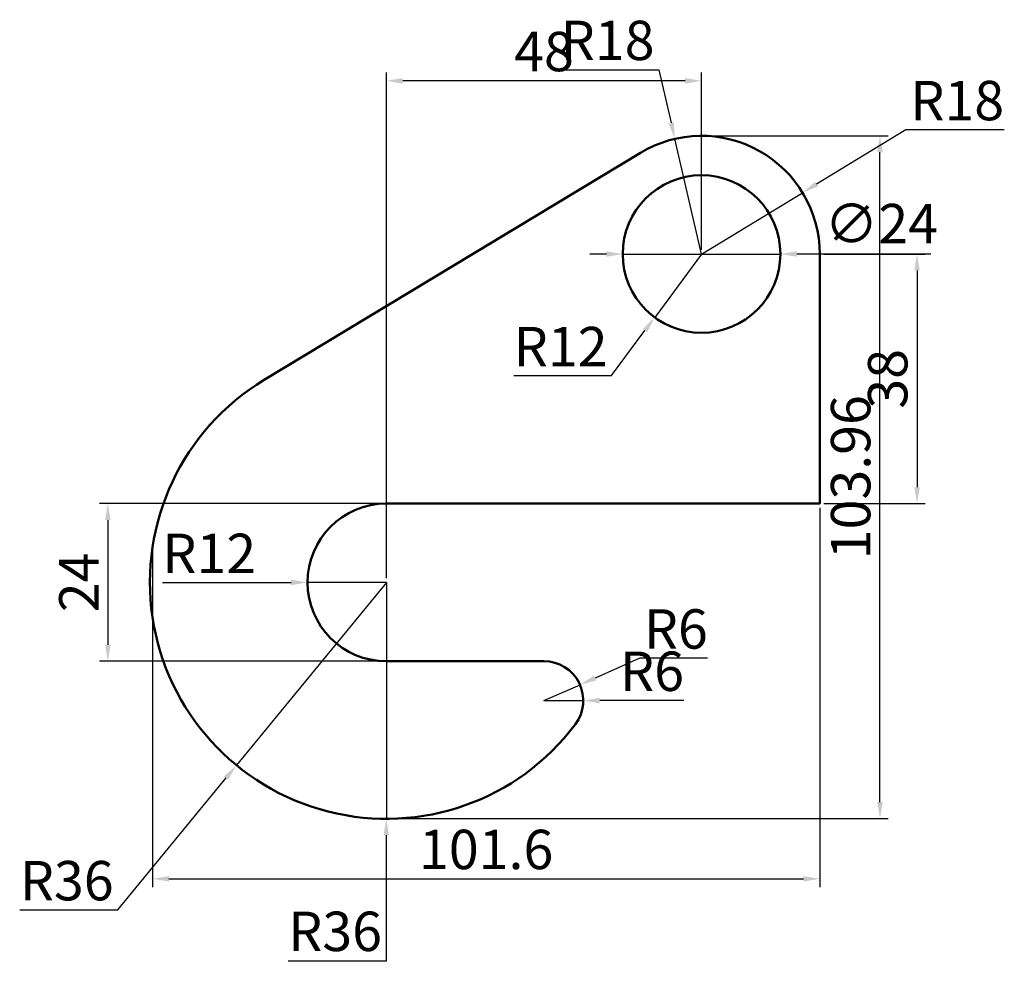
# Model space of a CAD drawing. Units: millimetres. Extents: x 135 to 285, y 18 to 161.
import ezdxf

# ---------------------------------------------------------------- set-up
doc = ezdxf.new("R2010")
doc.units = ezdxf.units.MM
doc.layers.add('M-DIMS', color=2, linetype='Continuous', lineweight=25)
doc.layers.add('M-OUTL', color=7, linetype='Continuous', lineweight=50)
doc.styles.get("Standard").update_dxf_attribs({"font": 'arial.ttf'})
doc.dimstyles.new('ISO-25', dxfattribs={"dimtxt": 6, "dimasz": 2.5, "dimexe": 1.25, "dimexo": 0.625, "dimtad": 1, "dimtoh": 1, "dimdec": 0, "dimtxsty": 'Standard', "dimcen": 2.5, "dimadec": 0, "dimazin": 0, "dimtfac": 1, "dimtdec": 0, "dimtmove": 0, "dimatfit": 3, "dimfxl": 1, "dimarcsym": 0})

# ---------------------------------------------------------------- blocks, each defined once
blk = doc.blocks.new('*D1')
at = {"layer": 'Defpoints', "color": 0, "transparency": 16777216}
for p in [(191.17, 87.46), (148.76, 63.46), (191.17, 63.46)]:
    blk.add_point(p, dxfattribs=at)
at = {"layer": 'M-DIMS', "color": 0, "lineweight": -2, "transparency": 16777216}
for p, q in [((190.54, 87.46), (147.51, 87.46)), ((148.76, 84.96), (148.76, 65.96)), ((190.54, 63.46), (147.51, 63.46))]:
    blk.add_line(p, q, dxfattribs=at)
at = {"layer": 'M-DIMS', "color": 0, "transparency": 16777216}
for points in [[(148.34, 84.96), (149.18, 84.96), (148.76, 87.46)], [(148.34, 65.96), (149.18, 65.96), (148.76, 63.46)]]:
    blk.add_solid(points, dxfattribs=at)
at = {"layer": 'M-DIMS', "color": 0, "transparency": 16777216, "insert": (145.12, 75.46), "char_height": 6, "attachment_point": 5, "rotation": 90}
blk.add_mtext('24', dxfattribs=at)
blk = doc.blocks.new('*D2')
at = {"layer": 'Defpoints', "color": 0, "transparency": 16777216}
for p in [(191.17, 75.46), (168.35, 47.61)]:
    blk.add_point(p, dxfattribs=at)
at = {"layer": 'M-DIMS', "color": 0, "lineweight": -2, "transparency": 16777216}
for p, q in [((191.17, 75.46), (168.35, 47.61)), ((150.3, 25.58), (166.77, 45.68)), ((135.34, 25.58), (150.3, 25.58))]:
    blk.add_line(p, q, dxfattribs=at)
at = {"layer": 'M-DIMS', "color": 0, "transparency": 16777216}
blk.add_solid([(166.44, 45.94), (167.09, 45.42), (168.35, 47.61)], dxfattribs=at)
at = {"layer": 'M-DIMS', "color": 0, "transparency": 16777216, "insert": (142.5, 29.27), "char_height": 6, "attachment_point": 5}
blk.add_mtext('R36', dxfattribs=at)
blk = doc.blocks.new('*D3')
at = {"layer": 'Defpoints', "color": 0, "transparency": 16777216}
for p in [(191.17, 151.83), (239.17, 125.46), (191.17, 75.46)]:
    blk.add_point(p, dxfattribs=at)
at = {"layer": 'M-DIMS', "color": 0, "lineweight": -2, "transparency": 16777216}
for p, q in [((191.17, 76.09), (191.17, 153.08)), ((239.17, 126.09), (239.17, 153.08)), ((236.67, 151.83), (193.67, 151.83))]:
    blk.add_line(p, q, dxfattribs=at)
at = {"layer": 'M-DIMS', "color": 0, "transparency": 16777216}
for points in [[(193.67, 152.25), (193.67, 151.41), (191.17, 151.83)], [(236.67, 152.25), (236.67, 151.41), (239.17, 151.83)]]:
    blk.add_solid(points, dxfattribs=at)
at = {"layer": 'M-DIMS', "color": 0, "transparency": 16777216, "insert": (215.17, 155.52), "char_height": 6, "attachment_point": 5}
blk.add_mtext('48', dxfattribs=at)
blk = doc.blocks.new('*D4')
at = {"layer": 'Defpoints', "color": 0, "transparency": 16777216}
for p in [(239.17, 125.46), (232.03, 115.81)]:
    blk.add_point(p, dxfattribs=at)
at = {"layer": 'M-DIMS', "color": 0, "lineweight": -2, "transparency": 16777216}
for p, q in [((239.17, 125.46), (232.03, 115.81)), ((225.47, 106.95), (230.54, 113.8)), ((210.57, 106.95), (225.47, 106.95))]:
    blk.add_line(p, q, dxfattribs=at)
at = {"layer": 'M-DIMS', "color": 0, "transparency": 16777216}
blk.add_solid([(230.21, 114.05), (230.88, 113.56), (232.03, 115.81)], dxfattribs=at)
at = {"layer": 'M-DIMS', "color": 0, "transparency": 16777216, "insert": (217.71, 110.59), "char_height": 6, "attachment_point": 5}
blk.add_mtext('R12', dxfattribs=at)
blk = doc.blocks.new('*D5')
at = {"layer": 'Defpoints', "color": 0, "transparency": 16777216}
for p in [(254.55, 134.8), (239.17, 125.46)]:
    blk.add_point(p, dxfattribs=at)
at = {"layer": 'M-DIMS', "color": 0, "lineweight": -2, "transparency": 16777216}
for p, q in [((270.3, 144.36), (256.69, 136.1)), ((285.27, 144.36), (270.3, 144.36)), ((239.17, 125.46), (254.55, 134.8))]:
    blk.add_line(p, q, dxfattribs=at)
at = {"layer": 'M-DIMS', "color": 0, "transparency": 16777216}
blk.add_solid([(256.47, 136.46), (256.91, 135.74), (254.55, 134.8)], dxfattribs=at)
at = {"layer": 'M-DIMS', "color": 0, "transparency": 16777216, "insert": (278.1, 148.05), "char_height": 6, "attachment_point": 5}
blk.add_mtext('R18', dxfattribs=at)
blk = doc.blocks.new('*D6')
at = {"layer": 'Defpoints', "color": 0, "transparency": 16777216}
for p in [(257.17, 125.46), (257.17, 87.46), (271.98, 87.46)]:
    blk.add_point(p, dxfattribs=at)
at = {"layer": 'M-DIMS', "color": 0, "lineweight": -2, "transparency": 16777216}
for p, q in [((257.79, 125.46), (273.23, 125.46)), ((271.98, 122.96), (271.98, 89.96)), ((257.79, 87.46), (273.23, 87.46))]:
    blk.add_line(p, q, dxfattribs=at)
at = {"layer": 'M-DIMS', "color": 0, "transparency": 16777216}
for points in [[(271.57, 122.96), (272.4, 122.96), (271.98, 125.46)], [(271.57, 89.96), (272.4, 89.96), (271.98, 87.46)]]:
    blk.add_solid(points, dxfattribs=at)
at = {"layer": 'M-DIMS', "color": 0, "transparency": 16777216, "insert": (268.29, 106.46), "char_height": 6, "attachment_point": 5, "rotation": 90}
blk.add_mtext('38', dxfattribs=at)
blk = doc.blocks.new('*D7')
at = {"layer": 'Defpoints', "color": 0, "transparency": 16777216}
for p in [(220.66, 59.88), (215.17, 57.46)]:
    blk.add_point(p, dxfattribs=at)
at = {"layer": 'M-DIMS', "color": 0, "lineweight": -2, "transparency": 16777216}
for p, q in [((229.79, 63.9), (222.95, 60.89)), ((240.09, 63.9), (229.79, 63.9)), ((215.17, 57.46), (220.66, 59.88))]:
    blk.add_line(p, q, dxfattribs=at)
at = {"layer": 'M-DIMS', "color": 0, "transparency": 16777216}
blk.add_solid([(222.78, 61.27), (223.11, 60.51), (220.66, 59.88)], dxfattribs=at)
at = {"layer": 'M-DIMS', "color": 0, "transparency": 16777216, "insert": (235.25, 67.59), "char_height": 6, "attachment_point": 5}
blk.add_mtext('R6', dxfattribs=at)
blk = doc.blocks.new('*D8')
at = {"layer": 'Defpoints', "color": 0, "transparency": 16777216}
for p in [(238.9, 143.46), (266.34, 143.46), (192.93, 39.5)]:
    blk.add_point(p, dxfattribs=at)
at = {"layer": 'M-DIMS', "color": 0, "lineweight": -2, "transparency": 16777216}
for p, q in [((239.53, 143.46), (267.59, 143.46)), ((266.34, 42), (266.34, 140.96)), ((193.55, 39.5), (267.59, 39.5))]:
    blk.add_line(p, q, dxfattribs=at)
at = {"layer": 'M-DIMS', "color": 0, "transparency": 16777216}
for points in [[(265.92, 140.96), (266.76, 140.96), (266.34, 143.46)], [(265.92, 42), (266.76, 42), (266.34, 39.5)]]:
    blk.add_solid(points, dxfattribs=at)
at = {"layer": 'M-DIMS', "color": 0, "transparency": 16777216, "insert": (262.65, 91.48), "char_height": 6, "attachment_point": 5, "rotation": 90}
blk.add_mtext('103.96', dxfattribs=at)
blk = doc.blocks.new('*D9')
at = {"layer": 'Defpoints', "color": 0, "transparency": 16777216}
for p in [(257.17, 87.46), (155.57, 80.82), (257.17, 30.33)]:
    blk.add_point(p, dxfattribs=at)
at = {"layer": 'M-DIMS', "color": 0, "lineweight": -2, "transparency": 16777216}
for p, q in [((257.17, 86.84), (257.17, 29.08)), ((155.57, 80.19), (155.57, 29.08)), ((158.07, 30.33), (254.67, 30.33))]:
    blk.add_line(p, q, dxfattribs=at)
at = {"layer": 'M-DIMS', "color": 0, "transparency": 16777216}
for points in [[(158.07, 30.74), (158.07, 29.91), (155.57, 30.33)], [(254.67, 30.74), (254.67, 29.91), (257.17, 30.33)]]:
    blk.add_solid(points, dxfattribs=at)
at = {"layer": 'M-DIMS', "color": 0, "transparency": 16777216, "insert": (206.37, 34.02), "char_height": 6, "attachment_point": 5}
blk.add_mtext('101.6', dxfattribs=at)
blk = doc.blocks.new('*D10')
at = {"layer": 'Defpoints', "color": 0, "transparency": 16777216}
for p in [(235.1, 143), (239.17, 125.46)]:
    blk.add_point(p, dxfattribs=at)
at = {"layer": 'M-DIMS', "color": 0, "lineweight": -2, "transparency": 16777216}
for p, q in [((217.69, 153.52), (232.66, 153.52)), ((232.66, 153.52), (234.54, 145.43)), ((239.17, 125.46), (235.1, 143))]:
    blk.add_line(p, q, dxfattribs=at)
at = {"layer": 'M-DIMS', "color": 0, "transparency": 16777216}
blk.add_solid([(234.94, 145.53), (234.13, 145.34), (235.1, 143)], dxfattribs=at)
at = {"layer": 'M-DIMS', "color": 0, "transparency": 16777216, "insert": (224.86, 157.21), "char_height": 6, "attachment_point": 5}
blk.add_mtext('R18', dxfattribs=at)
blk = doc.blocks.new('*D11')
at = {"layer": 'Defpoints', "color": 0, "transparency": 16777216}
for p in [(227.17, 125.46), (251.17, 125.46)]:
    blk.add_point(p, dxfattribs=at)
at = {"layer": 'M-DIMS', "color": 0, "lineweight": -2, "transparency": 16777216}
for p, q in [((224.67, 125.46), (222.17, 125.46)), ((227.17, 125.46), (251.17, 125.46)), ((258.37, 125.46), (253.67, 125.46)), ((274.09, 125.46), (258.37, 125.46))]:
    blk.add_line(p, q, dxfattribs=at)
at = {"layer": 'M-DIMS', "color": 0, "transparency": 16777216}
for points in [[(224.67, 125.88), (224.67, 125.04), (227.17, 125.46)], [(253.67, 125.88), (253.67, 125.04), (251.17, 125.46)]]:
    blk.add_solid(points, dxfattribs=at)
at = {"layer": 'M-DIMS', "color": 0, "transparency": 16777216, "insert": (266.54, 129.32), "char_height": 6, "attachment_point": 5}
blk.add_mtext('∅24', dxfattribs=at)
blk = doc.blocks.new('*D12')
at = {"layer": 'Defpoints', "color": 0, "transparency": 16777216}
for p in [(179.17, 75.46), (191.17, 75.46)]:
    blk.add_point(p, dxfattribs=at)
at = {"layer": 'M-DIMS', "color": 0, "lineweight": -2, "transparency": 16777216}
for p, q in [((157.07, 75.46), (171.97, 75.46)), ((171.97, 75.46), (176.67, 75.46)), ((191.17, 75.46), (179.17, 75.46))]:
    blk.add_line(p, q, dxfattribs=at)
at = {"layer": 'M-DIMS', "color": 0, "transparency": 16777216}
blk.add_solid([(176.67, 75.88), (176.67, 75.04), (179.17, 75.46)], dxfattribs=at)
at = {"layer": 'M-DIMS', "color": 0, "transparency": 16777216, "insert": (164.2, 79.1), "char_height": 6, "attachment_point": 5}
blk.add_mtext('R12', dxfattribs=at)
blk = doc.blocks.new('*D13')
at = {"layer": 'Defpoints', "color": 0, "transparency": 16777216}
for p in [(215.17, 57.46), (221.17, 57.46)]:
    blk.add_point(p, dxfattribs=at)
at = {"layer": 'M-DIMS', "color": 0, "lineweight": -2, "transparency": 16777216}
for p, q in [((215.17, 57.46), (221.17, 57.46)), ((226.17, 57.46), (223.67, 57.46)), ((236.46, 57.46), (226.17, 57.46))]:
    blk.add_line(p, q, dxfattribs=at)
at = {"layer": 'M-DIMS', "color": 0, "transparency": 16777216}
blk.add_solid([(223.67, 57.88), (223.67, 57.04), (221.17, 57.46)], dxfattribs=at)
at = {"layer": 'M-DIMS', "color": 0, "transparency": 16777216, "insert": (231.63, 61.15), "char_height": 6, "attachment_point": 5}
blk.add_mtext('R6', dxfattribs=at)
blk = doc.blocks.new('*D14')
at = {"layer": 'Defpoints', "color": 0, "transparency": 16777216}
for p in [(191.17, 75.46), (191.17, 39.46)]:
    blk.add_point(p, dxfattribs=at)
at = {"layer": 'M-DIMS', "color": 0, "lineweight": -2, "transparency": 16777216}
for p, q in [((191.17, 75.46), (191.17, 39.46)), ((191.17, 17.86), (191.17, 36.96)), ((176.21, 17.86), (191.17, 17.86))]:
    blk.add_line(p, q, dxfattribs=at)
at = {"layer": 'M-DIMS', "color": 0, "transparency": 16777216}
blk.add_solid([(190.75, 36.96), (191.58, 36.96), (191.17, 39.46)], dxfattribs=at)
at = {"layer": 'M-DIMS', "color": 0, "transparency": 16777216, "insert": (183.37, 21.55), "char_height": 6, "attachment_point": 5}
blk.add_mtext('R36', dxfattribs=at)

msp = doc.modelspace()

# ---------------------------------------------------------------- linework, layer by layer
at = {"layer": 'M-OUTL'}
msp.add_lwpolyline([(172.562, 106.281), (229.864, 140.871, -0.5838666), (257.166, 125.461), (257.166, 87.461), (191.166, 87.461, 1), (191.166, 63.461), (215.166, 63.461, -0.618034), (219.966, 53.861, -1.2132393)], format="xyb", close=True, dxfattribs=at)
msp.add_circle((239.166, 125.461), 12, dxfattribs=at)

# ---------------------------------------------------------------- dimensions: what is measured, and where the dimension line sits
at = {"layer": 'M-DIMS'}
for center, mpoint, override, picture, middle in [((239.166, 125.461), (235.101, 142.996), {"dimdec": 0, "dimlfac": 1, "dimrnd": 0, "dimzin": 0, "dimdsep": 46, "dimlunit": 2}, '*D10', (224.862, 153.517)), ((239.166, 125.461), (254.553, 134.802), {"dimclrd": 0, "dimclre": 0, "dimclrt": 0}, '*D5', (278.096, 144.361)), ((191.166, 75.461), (179.166, 75.461), {"dimdec": 0, "dimlfac": 1, "dimrnd": 0, "dimzin": 0, "dimdsep": 46, "dimlunit": 2}, '*D12', (171.966, 75.461)), ((191.166, 75.461), (168.351, 47.614), {"dimclrd": 0, "dimclre": 0, "dimclrt": 0}, '*D2', (142.504, 25.578)), ((191.166, 75.461), (191.166, 39.461), {"dimdec": 0, "dimlfac": 1, "dimrnd": 0, "dimzin": 0, "dimdsep": 46, "dimlunit": 2}, '*D14', (183.374, 17.861)), ((215.166, 57.461), (220.657, 59.879), {"dimclrd": 0, "dimclre": 0, "dimclrt": 0}, '*D7', (235.252, 63.903))]:
    dim = msp.add_radius_dim(center=center, mpoint=mpoint, dimstyle='ISO-25', override=override, dxfattribs=at)
    dim.commit()
    dim.dimension.update_dxf_attribs({"geometry": picture, "text_midpoint": middle, "dimtype": 164})
for base, p1, p2, override, picture, middle in [((191.166, 151.829), (239.166, 125.461), (191.166, 75.461), {"dimclrd": 0, "dimclre": 0, "dimclrt": 0}, '*D3', (215.166, 155.518)), ((257.166, 30.327), (155.565, 80.816), (257.166, 87.461), {"dimdec": 1, "dimlfac": 1, "dimrnd": 0, "dimzin": 0, "dimdsep": 46, "dimlunit": 2}, '*D9', (206.366, 34.016))]:
    dim = msp.add_linear_dim(base=base, p1=p1, p2=p2, dimstyle='ISO-25', override=override, dxfattribs=at)
    dim.commit()
    dim.dimension.update_dxf_attribs({"geometry": picture, "text_midpoint": middle})
for base, p1, p2, override, picture, middle in [((266.341, 143.459), (192.925, 39.502), (238.903, 143.459), {"dimdec": 2, "dimlfac": 1, "dimrnd": 0, "dimzin": 0, "dimdsep": 46, "dimlunit": 2}, '*D8', (262.651, 91.481)), ((271.984, 87.461), (257.166, 125.461), (257.166, 87.461), {"dimclrd": 0, "dimclre": 0, "dimclrt": 0}, '*D6', (268.294, 106.461)), ((148.759, 63.461), (191.166, 87.461), (191.166, 63.461), {"dimclrd": 0, "dimclre": 0, "dimclrt": 0}, '*D1', (145.121, 75.461))]:
    dim = msp.add_linear_dim(base=base, p1=p1, p2=p2, angle=90, dimstyle='ISO-25', override=override, dxfattribs=at)
    dim.commit()
    dim.dimension.update_dxf_attribs({"geometry": picture, "text_midpoint": middle})
dim = msp.add_diameter_dim_2p(p1=(227.166, 125.461), p2=(251.166, 125.461), dimstyle='ISO-25', override={"dimdec": 0, "dimlfac": 1, "dimrnd": 0, "dimzin": 0, "dimdsep": 46, "dimlunit": 2}, dxfattribs=at)
dim.commit()
dim.dimension.update_dxf_attribs({"geometry": '*D11', "text_midpoint": (258.366, 125.461), "dimtype": 163})
for center, mpoint, override, picture, middle in [((239.166, 125.461), (232.029, 115.814), {"dimclrd": 0, "dimclre": 0, "dimclrt": 0}, '*D4', (217.709, 110.589)), ((215.166, 57.461), (221.166, 57.461), {"dimdec": 0, "dimlfac": 1, "dimrnd": 0, "dimzin": 0, "dimdsep": 46, "dimlunit": 2}, '*D13', (231.627, 61.15))]:
    dim = msp.add_radius_dim(center=center, mpoint=mpoint, dimstyle='ISO-25', override=override, dxfattribs=at)
    dim.commit()
    dim.dimension.update_dxf_attribs({"geometry": picture, "text_midpoint": middle})

doc.saveas('drawing.dxf')
